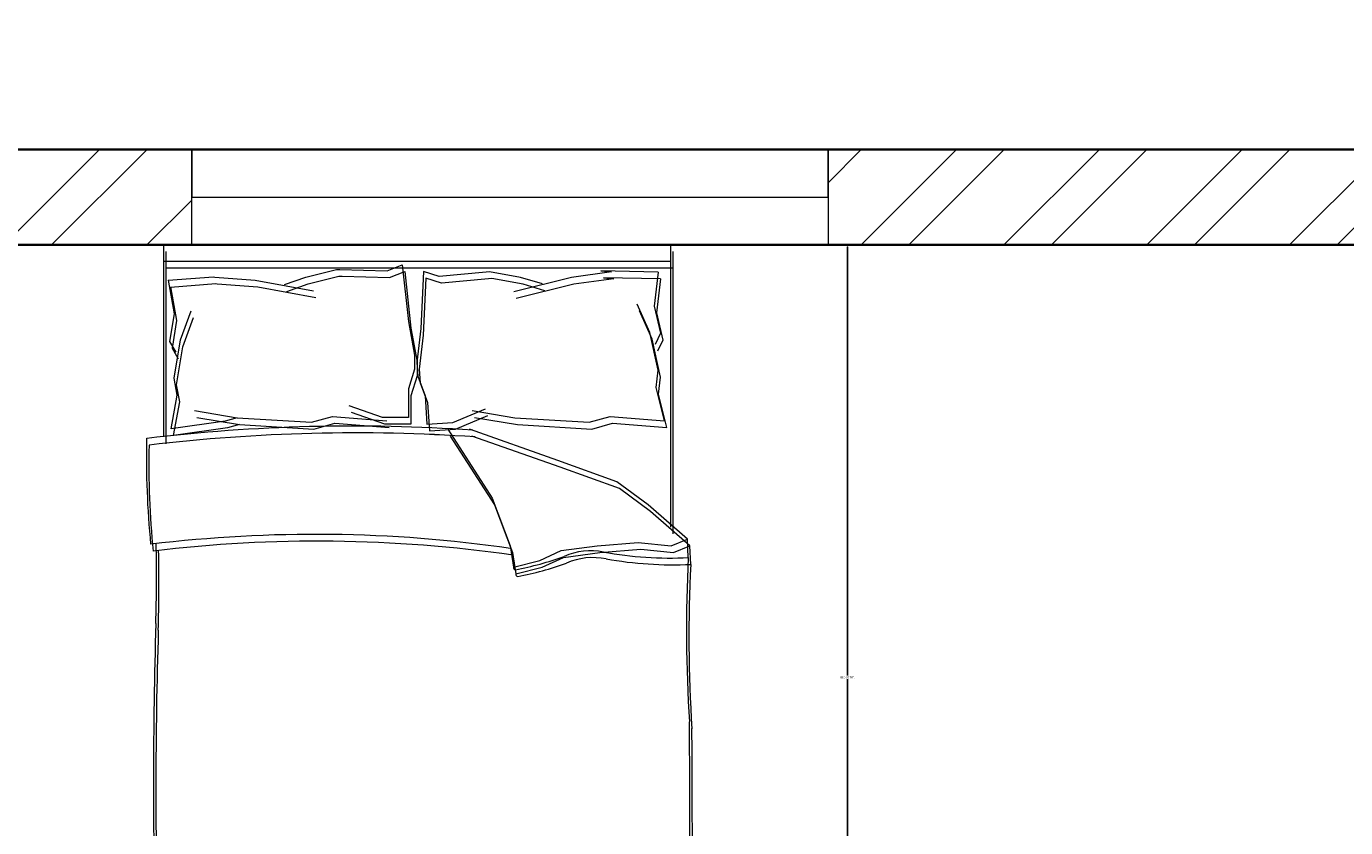
# Model space of a CAD drawing. Units: inches. Extents: x 2120 to 4013, y 1390 to 3019.
# Tile 41 of 59: x 2736 to 2861, y 2289 to 2364. Entities that reach past the tile are written whole.
import ezdxf

# ---------------------------------------------------------------- set-up
doc = ezdxf.new("R2010")
doc.units = ezdxf.units.IN
for name, color, linetype, lineweight in [('A-ANNO-DIMS', 2, 'Continuous', 18), ('A-FURN', 8, 'Continuous', 13), ('A-GLAZ', 4, 'Continuous', 18), ('A-WALL', 7, 'Continuous', 35), ('A-WALL-PATT', 252, 'Continuous', 13)]:
    doc.layers.add(name, color=color, linetype=linetype, lineweight=lineweight)
doc.styles.get("Standard").update_dxf_attribs({"font": 'arial.ttf'})
doc.dimstyles.get("Standard").update_dxf_attribs({"dimtxt": 0.18, "dimasz": 0.18, "dimexe": 0.18, "dimexo": 0.0625, "dimgap": 0.09, "dimtad": 0, "dimtih": 1, "dimtoh": 1, "dimdec": 4, "dimzin": 0, "dimdsep": 46, "dimtxsty": 'Standard', "dimcen": 0.09, "dimadec": 0, "dimazin": 0, "dimtfac": 1, "dimtdec": 4, "dimtofl": 0, "dimtmove": 0, "dimatfit": 3, "dimfxl": 1, "dimtolj": 1, "dimtzin": 0, "dimarcsym": 0})

# ---------------------------------------------------------------- blocks, each defined once
blk = doc.blocks.new('BED-DOUBLE-PLAN')
for p, q in [((3.48, 63.34), (3.48, 81.45)), ((3.48, 81.45), (51.27, 81.45)), ((51.27, 81.45), (51.27, 54.84)), ((3.48, 79.91), (51.27, 79.91)), ((3.7, 62.7), (3.7, 80.81)), ((51.5, 80.81), (51.5, 54.2)), ((3.7, 79.27), (51.5, 79.27)), ((3.9, 78.11), (8.18, 78.44)), ((8.18, 78.44), (8.29, 78.42)), ((8.29, 78.42), (12.11, 78.13)), ((14.86, 77.7), (16.88, 78.42)), ((16.88, 78.42), (19.77, 79.14)), ((17.11, 77.78), (20, 78.5)), ((19.77, 79.14), (20.09, 79.14)), ((20, 78.5), (20.32, 78.5)), ((20.09, 79.14), (24.54, 79)), ((20.32, 78.5), (24.77, 78.36)), ((24.54, 79), (25.98, 79.58)), ((24.77, 78.36), (26.21, 78.94)), ((25.98, 79.58), (26.56, 74.23)), ((26.21, 78.94), (26.79, 73.59)), ((27.98, 78.95), (27.73, 73.58)), ((29.46, 78.47), (27.98, 78.95)), ((33.89, 78.89), (29.46, 78.47)), ((34.21, 78.91), (33.89, 78.89)), ((37.14, 78.37), (34.21, 78.91)), ((41.92, 78.38), (36.5, 77.02)), ((45.71, 78.9), (41.92, 78.38)), ((50.11, 78.89), (44.71, 78.99)), ((44.71, 78.99), (45.71, 78.9)), ((50.11, 78.89), (49.73, 75.68)), ((3.9, 78.13), (4.47, 74.95)), ((4.12, 77.49), (4.7, 74.31)), ((4.13, 77.47), (8.41, 77.8)), ((8.41, 77.8), (8.51, 77.78)), ((8.51, 77.78), (12.34, 77.49)), ((12.11, 78.13), (17.6, 77.12)), ((12.34, 77.49), (17.83, 76.48)), ((15.08, 77.06), (17.11, 77.78)), ((28.21, 78.32), (27.96, 72.94)), ((29.69, 77.83), (28.21, 78.32)), ((34.11, 78.25), (29.69, 77.83)), ((34.43, 78.27), (34.11, 78.25)), ((37.37, 77.73), (34.43, 78.27)), ((42.14, 77.74), (36.72, 76.38)), ((39.2, 77.77), (37.14, 78.37)), ((39.43, 77.13), (37.37, 77.73)), ((45.94, 78.26), (42.14, 77.74)), ((50.34, 78.25), (44.94, 78.35)), ((44.94, 78.35), (45.94, 78.26)), ((50.34, 78.25), (49.96, 75.04)), ((4.47, 74.95), (4.04, 72.35)), ((5.05, 72.49), (6.06, 75.24)), ((49.31, 73.19), (48.13, 75.87)), ((49.54, 72.55), (48.36, 75.23)), ((49.73, 75.68), (50.33, 73.11)), ((49.96, 75.04), (50.56, 72.47)), ((4.7, 74.31), (4.27, 71.71)), ((5.28, 71.85), (6.29, 74.6)), ((26.56, 74.23), (27.14, 71.05)), ((26.79, 73.59), (27.37, 70.41)), ((27.73, 73.58), (27.36, 70.37)), ((4.04, 72.35), (4.62, 71.33)), ((4.47, 68.88), (5.05, 72.49)), ((27.96, 72.94), (27.58, 69.73)), ((50.11, 69.62), (49.31, 73.19)), ((50.34, 68.98), (49.54, 72.55)), ((50.33, 73.11), (49.82, 72.06)), ((50.56, 72.47), (50.04, 71.42)), ((4.27, 71.71), (4.85, 70.7)), ((4.7, 68.24), (5.28, 71.85)), ((27.14, 71.05), (27.14, 69.74)), ((27.14, 69.74), (26.56, 67.86)), ((27.36, 70.37), (27.44, 69.07)), ((27.37, 70.41), (27.37, 69.1)), ((27.58, 69.73), (27.67, 68.43)), ((4.76, 67.29), (4.47, 68.88)), ((27.37, 69.1), (26.79, 67.23)), ((27.44, 69.07), (28.13, 67.23)), ((27.67, 68.43), (28.36, 66.59)), ((49.92, 68.01), (50.11, 69.62)), ((50.15, 67.37), (50.34, 68.98)), ((4.19, 64.11), (4.76, 67.29)), ((4.99, 66.65), (4.7, 68.24)), ((26.56, 67.86), (26.56, 65.18)), ((26.79, 67.23), (26.79, 64.54)), ((28.13, 67.23), (28.3, 64.55)), ((50.7, 64.87), (49.92, 68.01)), ((50.93, 64.23), (50.15, 67.37)), ((4.41, 63.47), (4.99, 66.65)), ((24.1, 65.18), (20.96, 66.27)), ((28.36, 66.59), (28.53, 63.91)), ((30.75, 64.71), (33.82, 65.99)), ((9.28, 64.83), (4.19, 64.11)), ((6.38, 65.82), (10.42, 65.15)), ((6.61, 65.18), (10.64, 64.51)), ((10.42, 65.15), (9.28, 64.83)), ((10.42, 65.15), (17.43, 64.72)), ((17.43, 64.72), (19.39, 65.28)), ((19.39, 65.28), (24.52, 64.87)), ((24.33, 64.54), (21.19, 65.63)), ((26.56, 65.18), (24.1, 65.18)), ((28.3, 64.55), (30.75, 64.71)), ((30.98, 64.07), (34.05, 65.35)), ((32.57, 65.82), (36.6, 65.15)), ((32.79, 65.18), (36.83, 64.51)), ((36.6, 65.15), (43.61, 64.72)), ((43.61, 64.72), (45.57, 65.28)), ((45.57, 65.28), (50.7, 64.87)), ((9.51, 64.19), (4.41, 63.47)), ((10.64, 64.51), (9.51, 64.19)), ((10.64, 64.51), (17.65, 64.08)), ((17.65, 64.08), (19.61, 64.64)), ((19.61, 64.64), (24.75, 64.23)), ((26.79, 64.54), (24.33, 64.54)), ((28.53, 63.91), (30.98, 64.07)), ((30.26, 64.06), (34.45, 57.57)), ((40.65, 61.13), (32.31, 64.06)), ((36.83, 64.51), (43.84, 64.08)), ((43.84, 64.08), (45.8, 64.64)), ((45.8, 64.64), (50.93, 64.23)), ((30.49, 63.42), (34.68, 56.93)), ((40.87, 60.49), (32.54, 63.42)), ((46.22, 59.12), (40.65, 61.13)), ((46.45, 58.48), (40.87, 60.49)), ((49.16, 56.95), (46.22, 59.12)), ((49.39, 56.31), (46.45, 58.48)), ((34.45, 57.57), (36.15, 53.08)), ((34.68, 56.93), (36.38, 52.44)), ((52.87, 53.7), (49.16, 56.95)), ((53.1, 53.06), (49.39, 56.31)), ((51.33, 53.08), (52.87, 53.7)), ((52.95, 51.96), (52.87, 53.7, 3.87)), ((36.15, 53.08), (36.46, 51.07)), ((36.38, 52.44), (36.69, 50.43)), ((38.94, 51.69), (40.96, 52.62)), ((40.96, 52.62), (44.36, 53.08)), ((41.18, 51.98), (44.59, 52.44)), ((44.36, 53.08), (48.23, 53.39)), ((44.59, 52.44), (48.46, 52.75)), ((48.23, 53.39), (51.33, 53.08)), ((48.46, 52.75), (51.56, 52.44)), ((51.56, 52.44), (53.1, 53.06)), ((53.18, 51.32), (53.1, 53.06, 3.87)), ((36.46, 51.07), (38.94, 51.69)), ((36.69, 50.43), (39.17, 51.05)), ((39.17, 51.05), (41.18, 51.98)), ((15.06, 2.2), (39.68, 2.2)), ((15.29, 1.56), (39.91, 1.56))]:
    blk.add_line(p, q)
for centre, radius, start, end in [((21.36, -100.61), 164.97, 86.0865, 96.7821), ((21.59, -101.25), 164.97, 86.0865, 96.7821), ((85.16, 61.35), 83.31, 178.7218, 185.604), ((85.39, 60.71), 83.31, 178.7218, 185.604), ((17.76, -74.87), 129.02, 81.7845, 96.9006), ((17.99, -75.51), 129.02, 81.7845, 96.9006), ((-167.31, 50.27), 170.11, 358.4762, 1.0082), ((-167.08, 49.63), 170.11, 358.4762, 1.0082), ((43.74, 46.38), 6.22, 78.6608, 113.7384), ((51.33, 88.1), 36.18, 259.8763, 272.5657), ((36.64, 51.01), 0.185, 160.2464, 271.1377), ((31.16, 79.96), 29.65, 280.6617, 289.8806), ((31.38, 79.32), 29.65, 280.6617, 289.8806), ((43.97, 45.74), 6.22, 78.6608, 113.7384), ((51.56, 87.46), 36.18, 259.8763, 272.5657), ((182.27, 45.13), 129.5, 176.9791, 183.8365), ((182.5, 44.49), 129.5, 176.9791, 183.8365), ((36.87, 50.37), 0.185, 160.2464, 271.1377), ((484.82, 30.83), 482.31, 178.2277, 181.7185), ((485.05, 30.19), 482.31, 178.2277, 181.7185), ((-4508.74, 13.62), 4561.86, 0.00217, 0.28689), ((-4508.51, 12.99), 4561.86, 0.00217, 0.28689), ((-26.9, 16.93), 29.63, 346.0648, 358.9113), ((-26.67, 16.29), 29.63, 346.0648, 358.9113), ((76.16, 12.78), 23.07, 177.4714, 206.4681), ((76.39, 12.14), 23.07, 177.4714, 206.4681), ((-21.66, 11.17), 23.56, 337.9751, 356.652), ((-21.43, 10.53), 23.56, 337.9751, 356.652), ((-17.22, 105.16), 106.46, 283.3832, 287.7053), ((-16.99, 104.52), 106.46, 283.3832, 287.7053), ((54.41, 2.58), 1.1, 242.6588, 356.02), ((1.09, 1.73), 1.09, 146.1736, 293.4781), ((1.32, 1.09), 1.09, 146.1736, 293.4781), ((21.43, -119.39), 121.76, 92.9958, 99.4091), ((21.66, -120.03), 121.76, 92.9958, 99.4091), ((41.15, -130.83), 133.04, 84.4998, 90.6351), ((41.38, -131.47), 133.04, 84.4998, 90.6351), ((54.64, 1.94), 1.1, 242.6588, 356.02)]:
    blk.add_arc(centre, radius, start, end)
blk = doc.blocks.new('WIN-PLAN-60IN-02')
for p, q in [((0, 0), (0, 9)), ((0, 9), (0, 4.5)), ((60, 4.5), (60, 9)), ((60, 9), (60, 0)), ((0, 4.5), (60, 4.5))]:
    blk.add_line(p, q)
blk = doc.blocks.new('*D73')
at = {"layer": 'A-ANNO-DIMS', "color": 0, "lineweight": -2, "transparency": 16777216}
for p, q in [((2801.55, 2343.53), (2813.9, 2343.53)), ((2813.72, 2343.35), (2813.72, 2302.94)), ((2813.72, 2262.16), (2813.72, 2302.57)), ((2801.55, 2261.98), (2813.9, 2261.98))]:
    blk.add_line(p, q, dxfattribs=at)
at = {"layer": 'A-ANNO-DIMS', "color": 0, "transparency": 16777216}
for points in [[(2813.69, 2343.35), (2813.75, 2343.35), (2813.72, 2343.53)], [(2813.69, 2262.16), (2813.75, 2262.16), (2813.72, 2261.98)]]:
    blk.add_solid(points, dxfattribs=at)
at = {"layer": 'Defpoints', "color": 0, "transparency": 16777216}
for p in [(2801.49, 2343.53), (2813.72, 2343.53), (2801.49, 2261.98)]:
    blk.add_point(p, dxfattribs=at)
at = {"layer": 'A-ANNO-DIMS', "color": 0, "transparency": 16777216, "insert": (2813.72, 2302.76), "char_height": 0.18, "attachment_point": 5}
blk.add_mtext('\\A1;BED 82 TYP.', dxfattribs=at)
blk = doc.blocks.new('*D211')
at = {"layer": 'A-ANNO-DIMS', "color": 0, "lineweight": -2, "transparency": 16777216}
for p, q in [((2262.73, 2352.59), (2262.73, 2397.71)), ((2262.91, 2397.53), (2635.95, 2397.53)), ((3009.55, 2397.53), (2636.52, 2397.53)), ((3009.73, 2352.59), (3009.73, 2397.71))]:
    blk.add_line(p, q, dxfattribs=at)
at = {"layer": 'A-ANNO-DIMS', "color": 0, "transparency": 16777216}
for points in [[(2262.91, 2397.56), (2262.91, 2397.5), (2262.73, 2397.53)], [(3009.55, 2397.56), (3009.55, 2397.5), (3009.73, 2397.53)]]:
    blk.add_solid(points, dxfattribs=at)
at = {"layer": 'Defpoints', "color": 0, "transparency": 16777216}
for p in [(3009.73, 2397.53), (2262.73, 2352.53), (3009.73, 2352.53)]:
    blk.add_point(p, dxfattribs=at)
at = {"layer": 'A-ANNO-DIMS', "color": 0, "transparency": 16777216, "insert": (2636.23, 2397.53), "char_height": 0.18, "attachment_point": 5}
blk.add_mtext('\\A1;747', dxfattribs=at)

msp = doc.modelspace()

# ---------------------------------------------------------------- hatches: boundary and pattern name
at = {"layer": 'A-WALL-PATT'}
h = msp.add_hatch(dxfattribs=at)
h.set_pattern_fill('ANSI32', color=256)
h.paths.add_polyline_path([(2271.7331, 2122.6377), (2262.7331, 2122.6377), (2262.7331, 2040.3893), (2267.2331, 2040.3893), (2271.7331, 2040.3893), (2271.7331, 2044.8856), (2271.7331, 2070.531), (2391.7331, 2070.531), (2391.7331, 1926.5306), (2388.3993, 1926.5306), (2388.3993, 1922.531), (2395.7331, 1922.531), (2395.7331, 1992.531), (2400.4511, 1992.531), (2400.4511, 1997.0306), (2395.7331, 1997.0306), (2395.7331, 2070.531), (2443.7331, 2070.531), (2443.7331, 2046.1368), (2448.2331, 2046.1368), (2448.2331, 2070.531), (2580.2331, 2070.531), (2580.2331, 1997.0306), (2492.9076, 1997.0306), (2492.9076, 1992.531), (2580.2331, 1992.531), (2580.2331, 1983.9368), (2589.2331, 1983.9368), (2589.2331, 2070.531), (2589.2331, 2075.0306), (2396.2331, 2075.0306), (2396.2331, 2184.3565), (2393.9831, 2184.3565), (2391.7331, 2184.3565), (2391.7331, 2075.0306), (2271.7331, 2075.0306)])
h.paths.add_polyline_path([(2724.7331, 2138.0306), (2628.7331, 2138.0306), (2628.7331, 2070.5306), (2628.7331, 2067.0987), (2633.2331, 2067.0987), (2637.7331, 2067.0987), (2637.7331, 2070.531), (2657.3413, 2070.531), (2657.3413, 2079.5306), (2637.7331, 2079.5306), (2637.7331, 2129.031), (2715.7331, 2129.031), (2715.7331, 2079.5306), (2698.0378, 2079.5306), (2698.0378, 2070.531), (2715.7331, 2070.531), (2715.7331, 2012.1531), (2720.2331, 2012.1531), (2724.7331, 2012.1531)])
h.paths.add_polyline_path([(2724.7331, 2213.031), (2831.3209, 2213.031), (2831.3209, 2215.281), (2831.3209, 2217.5306), (2724.7331, 2217.5306), (2724.7331, 2343.531), (2751.8755, 2343.531), (2751.8755, 2352.5306), (2715.7331, 2352.5306), (2715.7331, 2138.031), (2724.7331, 2138.031)])
h.paths.add_polyline_path([(2902.53, 2352.5306), (2811.8755, 2352.5306), (2811.8755, 2343.531), (2867.2331, 2343.531), (2867.2331, 2217.5306), (2863.6364, 2217.5306), (2863.6364, 2213.031), (2871.7331, 2213.031), (2871.7331, 2217.531), (2871.7331, 2343.531), (2902.53, 2343.531)])
h.paths.add_polyline_path([(3009.7331, 2352.5306), (2938.53, 2352.5306), (2938.53, 2343.531), (2966.2331, 2343.531), (2966.2331, 2242.3281), (2968.4831, 2242.3281), (2970.7331, 2242.3281), (2970.7331, 2343.531), (3009.7331, 2343.531)])
h.paths.add_polyline_path([(3009.7331, 2217.5306), (2970.7331, 2217.5306), (2970.7331, 2220.5422), (2968.4831, 2220.5422), (2966.2331, 2220.5422), (2966.2331, 2217.5306), (2911.7752, 2217.5306), (2907.7331, 2217.5306), (2907.7331, 2213.0306), (2907.7331, 2194.9663), (2912.2331, 2194.9663), (2912.2331, 2213.031), (2970.7331, 2213.031), (3000.7331, 2213.031), (3000.7331, 2205.523), (3009.7331, 2205.523)])
h.paths.add_polyline_path([(3009.7331, 2181.5227), (3000.7331, 2181.5227), (3000.7331, 2165.0306), (2912.2331, 2165.0306), (2912.2331, 2170.8202), (2907.7331, 2170.8202), (2907.7331, 2165.0306), (2899.5169, 2165.0306), (2899.5169, 2162.7806), (2899.5169, 2160.531), (2907.7331, 2160.531), (2907.7331, 2137.3432), (2912.2331, 2137.3432), (2912.2331, 2160.531), (3000.7331, 2160.531), (3000.7331, 2150.4993), (3009.7331, 2150.4993)])
h.paths.add_polyline_path([(3009.7331, 2126.499), (3005.2331, 2126.499), (3000.7331, 2126.499), (3000.7331, 2112.5306), (2912.2331, 2112.5306), (2912.2331, 2115.6036), (2907.7331, 2115.6036), (2907.7331, 2108.031), (3000.7331, 2108.031), (3000.7331, 2084.7256), (3009.7331, 2084.7256)], flags=17)
h.paths.add_polyline_path([(3009.7331, 1971.531), (3009.7331, 2024.7253), (3000.7331, 2024.7253), (3000.7331, 2006.4153), (3000.7331, 1971.5306), (2864.2331, 1971.5306), (2864.2331, 2160.531), (2868.0522, 2160.531), (2868.0522, 2165.0306), (2859.7331, 2165.0306), (2859.7331, 1971.5306), (2724.7331, 1971.5306), (2724.7331, 1977.7012), (2715.7331, 1977.7012), (2715.7331, 1962.5306), (2715.7331, 1950.9035), (2720.2331, 1950.9035), (2724.7331, 1950.9035), (2724.7331, 1962.531), (2855.2331, 1962.531), (2859.7331, 1962.531), (2859.7331, 1835.031), (2864.2331, 1834.8158), (2864.2331, 1962.531), (2958.7331, 1962.531), (2958.7331, 1937.0925), (2963.2331, 1937.0925), (2963.2331, 1962.531), (3000.7331, 1962.531), (3009.7331, 1962.531)])
h.paths.add_polyline_path([(2724.7331, 1728.531), (2822.7164, 1728.531), (2822.7164, 1733.0306), (2724.7331, 1733.0306), (2724.7331, 1779.3416), (2715.7331, 1779.3416), (2715.7331, 1581.531), (2753.02, 1581.531), (2753.02, 1586.031), (2753.02, 1590.5306), (2724.7331, 1590.5306)])
h.paths.add_polyline_path([(2864.2331, 1590.531), (2864.2331, 1787.031), (2868.4075, 1787.031), (2868.4075, 1791.5306), (2859.7331, 1791.5306), (2859.7331, 1739.0306), (2859.7331, 1733.0306), (2854.3125, 1733.0306), (2854.3125, 1728.531), (2859.7331, 1728.531), (2859.7331, 1590.5306), (2813.02, 1590.5306), (2813.02, 1581.531), (2868.4123, 1581.531), (2868.4123, 1583.781), (2868.4123, 1586.0306), (2864.2331, 1586.0306)])
h.paths.add_polyline_path([(3009.7331, 1754.6619), (3000.7331, 1754.6619), (3000.7331, 1739.0306), (2912.2331, 1739.0306), (2912.2331, 1742.2257), (2907.7331, 1742.2257), (2907.7331, 1739.0306), (2907.7331, 1734.531), (3000.7331, 1734.531), (3000.7331, 1590.5306), (3000.7331, 1586.0306), (2971.3921, 1586.0306), (2971.3921, 1581.531), (3009.7331, 1581.531)])
h.paths.add_polyline_path([(2911.3921, 1583.781), (2911.3921, 1586.0306), (2891.2138, 1586.0306), (2891.2138, 1581.531), (2911.3921, 1581.531)])
h.paths.add_polyline_path([(3009.7331, 1799.8422), (3000.7331, 1799.8422), (3000.7331, 1791.5306), (2912.2331, 1791.5306), (2912.2331, 1796.3264), (2909.9831, 1796.3264), (2907.7331, 1796.3264), (2907.7331, 1791.5306), (2902.7033, 1791.5306), (2902.7033, 1787.031), (2907.7331, 1787.031), (2907.7331, 1761.1622), (2912.2331, 1761.1622), (2912.2331, 1787.031), (3000.7331, 1787.031), (3000.7331, 1778.6622), (3009.7331, 1778.6622)])
h.paths.add_polyline_path([(3009.7331, 1839.5306), (2963.2331, 1839.5306), (2963.2331, 1842.8629), (2960.9831, 1842.8629), (2958.7331, 1842.8629), (2958.7331, 1839.5306), (2907.7331, 1839.5306), (2907.7331, 1814.4599), (2912.2331, 1814.4599), (2912.2331, 1835.031), (3000.7331, 1835.031), (3000.7331, 1823.8425), (3009.7331, 1823.8425), (3009.7331, 1835.031)])
h.paths.add_polyline_path([(2963.2331, 1901.0922), (2960.9831, 1901.0922), (2958.7331, 1901.0922), (2958.7331, 1862.8843), (2963.2331, 1862.8843)], flags=17)
h.paths.add_polyline_path([(2724.7331, 1891.9826), (2724.7331, 1914.3416), (2715.7331, 1914.3416), (2715.7331, 1783.8416), (2637.7331, 1783.8416), (2637.7331, 1914.3416), (2628.7331, 1914.3416), (2624.7701, 1914.3416), (2624.7701, 1909.8416), (2624.7701, 1905.3419), (2628.7331, 1905.3419), (2628.7331, 1876.9915), (2628.7331, 1779.3419), (2637.7331, 1779.3419), (2715.7331, 1779.3419), (2724.7331, 1779.3419), (2724.7331, 1835.031)])
h.paths.add_polyline_path([(2637.7331, 1731.531), (2637.7331, 1779.3416), (2628.7331, 1779.3416), (2628.7331, 1731.5306), (2589.2331, 1731.5306), (2535.9814, 1731.5306), (2496.7331, 1731.5306), (2496.7331, 1725.6876), (2498.9831, 1725.6876), (2501.2331, 1725.6876), (2501.2331, 1727.031), (2628.7331, 1727.031), (2628.7331, 1680.4203), (2628.7331, 1590.5306), (2628.7331, 1586.0306), (2604.1361, 1586.0306), (2604.1361, 1581.531), (2637.7331, 1581.531), (2637.7331, 1590.531)])

# ---------------------------------------------------------------- linework, layer by layer
at = {"layer": 'A-WALL'}
for p, q in [((2715.7331, 2352.531), (3009.7331, 2352.531)), ((2715.7331, 2352.5306), (3009.7331, 2352.5306)), ((2724.7331, 2343.531), (2867.2331, 2343.531)), ((2724.7331, 2343.5306), (2867.2331, 2343.5306))]:
    msp.add_line(p, q, dxfattribs=at)

# ---------------------------------------------------------------- block references
at = {"layer": 'A-FURN'}
for p in [(2745.7528, 2262.0847), (2745.7528, 2262.0844)]:
    msp.add_blockref('BED-DOUBLE-PLAN', p, dxfattribs=at)
at = {"layer": 'A-GLAZ'}
for p in [(2751.8755, 2343.531), (2751.8755, 2343.5306)]:
    msp.add_blockref('WIN-PLAN-60IN-02', p, dxfattribs=at)

# ---------------------------------------------------------------- dimensions: what is measured, and where the dimension line sits
at = {"layer": 'A-ANNO-DIMS'}
dim = msp.add_linear_dim(base=(3009.7331, 2397.531), p1=(2262.7331, 2352.531), p2=(3009.7331, 2352.531), dimstyle='Standard', override={"dimdec": 0, "dimlfac": 1, "dimrnd": 0, "dimzin": 0, "dimdsep": 46, "dimlunit": 2}, dxfattribs=at)
dim.commit()
dim.dimension.update_dxf_attribs({"geometry": '*D211', "text_midpoint": (2636.2331, 2397.531)})
dim = msp.add_linear_dim(base=(2813.7246, 2343.531), p1=(2801.4923, 2261.9823), p2=(2801.4923, 2343.531), angle=90, text='BED <> TYP.', dimstyle='Standard', override={"dimdec": 0, "dimlfac": 1, "dimrnd": 0, "dimzin": 0, "dimdsep": 46, "dimlunit": 2}, dxfattribs=at)
dim.commit()
dim.dimension.update_dxf_attribs({"geometry": '*D73', "text_midpoint": (2813.7246, 2302.7566)})

doc.saveas('drawing.dxf')
